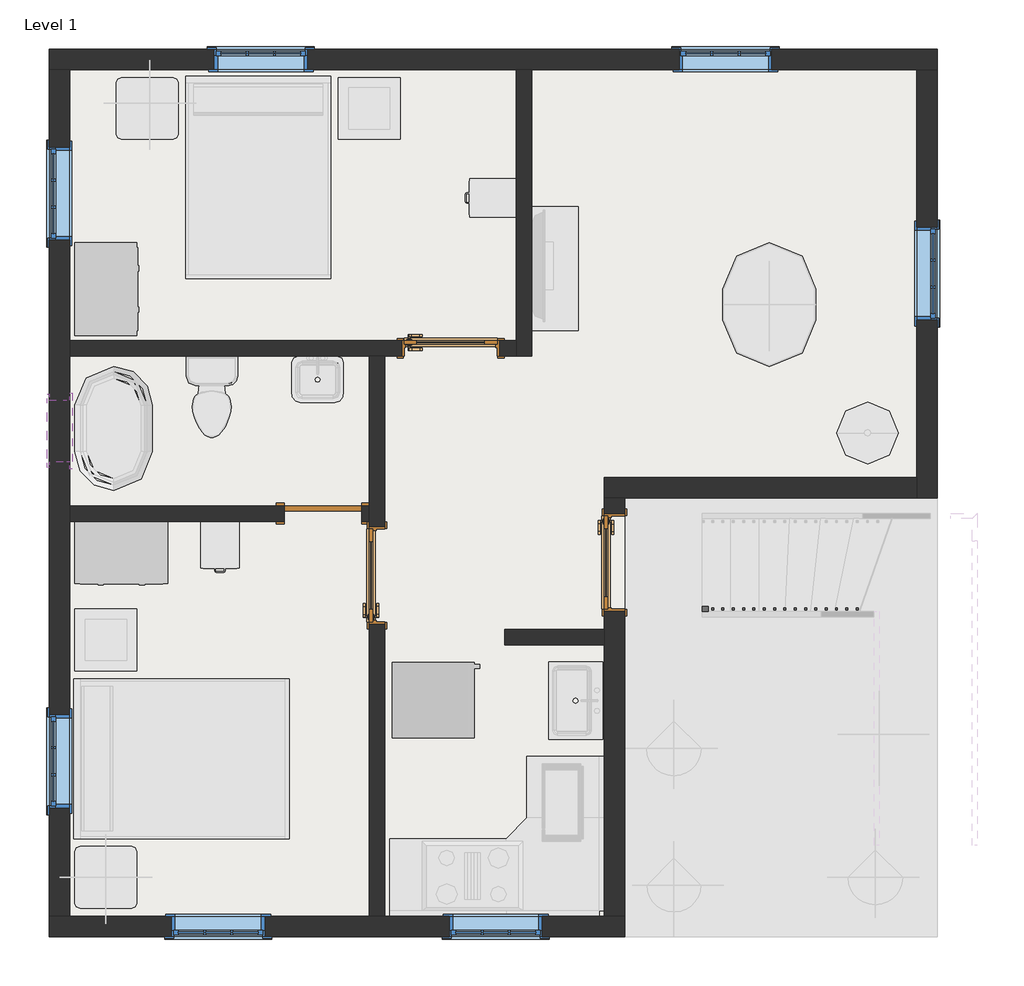
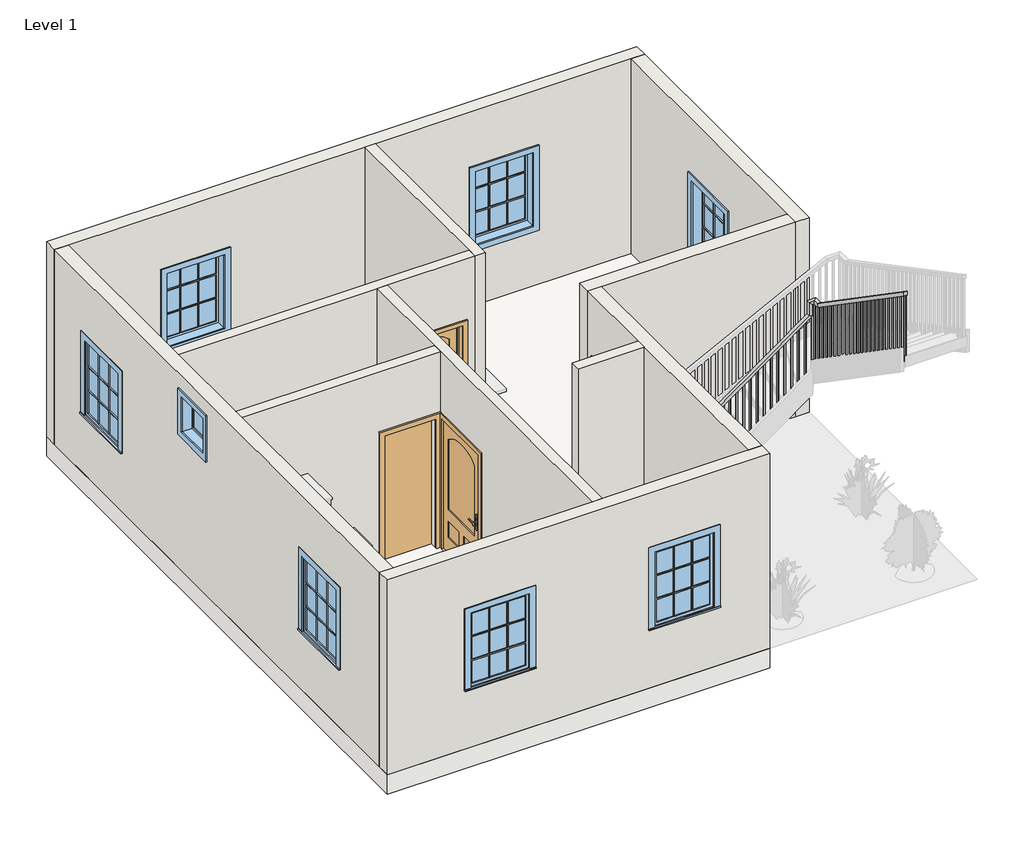
# One storey, part 1 of 2: 11 walls, 8 windows, 4 doors, 1 railing, 1 slab.
"""IFC4 building model written with IfcOpenShell, lengths in millimetres."""

from ifc_helpers import new_model, si_unit, frame, origin, origin_with_axes, place, context, project, spatial, polyline, outline, extrude, faceted_brep, transform, mapped, element, save
from components import door_5d363d20, door_1768e003, door_059fdd7e, window_29c06734, window_e41d21a6

model = new_model("IFC4")

# Units and contexts
model_context = context("Model", 3, world=origin())
ifc_project = project(units=[si_unit("LENGTHUNIT", "METRE", prefix="MILLI")], contexts=[model_context])

# Site, building, storey
site = spatial("IfcSite", under=ifc_project)
building = spatial("IfcBuilding", under=site)
storey = spatial("IfcBuildingStorey", under=building, Name="Level 1", Elevation=0.0)

# Doors
placement = place(None, origin())
door_shape = door_5d363d20(model_context)
element("IfcDoor", 1, ObjectType="36\" x 80\"", at=placement, inside=storey, context=model_context, shape_type="MappedRepresentation", body=[
    mapped(door_shape, transform((-9402.5770189, 12238.7273405, 0.0), x_axis=(-1.0, 0.0, 0.0), y_axis=(0.0, -1.0, 0.0), z_axis=(0.0, 0.0, 1.0))),
])
element("IfcDoor", 2, ObjectType="36\" x 80\"", at=placement, inside=storey, context=model_context, shape_type="MappedRepresentation", body=[
    mapped(door_shape, transform((-10129.6520189, 10000.3523405, 0.0), x_axis=(0.0, -1.0, 0.0), y_axis=(1.0, 0.0, 0.0), z_axis=(0.0, 0.0, 1.0))),
])
door_2_shape = door_1768e003(model_context)
element("IfcDoor", 3, ObjectType="36\" x 80\"", at=placement, inside=storey, context=model_context, shape_type="MappedRepresentation", body=[
    mapped(door_2_shape, transform((-7792.8520189, 10127.3523405, 0.0), x_axis=(0.0, 1.0, 0.0), y_axis=(-1.0, 0.0, 0.0), z_axis=(0.0, 0.0, 1.0))),
])
door_3_shape = door_059fdd7e(model_context)
element("IfcDoor", 4, ObjectType="Single-Flush : 30\" x 80\"", at=placement, inside=storey, context=model_context, shape_type="MappedRepresentation", body=[
    mapped(door_3_shape, transform((-10659.8770189, 10609.9523405, 0.0), x_axis=(1.0, 0.0, 0.0), y_axis=(0.0, 1.0, 0.0), z_axis=(0.0, 0.0, 1.0))),
])

# Railing
element("IfcRailing", 5, ObjectType="Handrail - Rectangular", at=placement, inside=storey, context=model_context, shape_type="SolidModel", body=[
    faceted_brep([(-6926.0770189, 9695.5523405, 1221.3337634), (-6926.0770189, 9695.5523405, 1158.7470985), (-6926.0770189, 9644.7523405, 1158.7470985), (-6926.0770189, 9644.7523405, 1221.3337634), (-5260.1400294, 9695.5523405, 2420.2016261), (-5209.3400294, 9695.5523405, 2394.1724587), (-5209.3400294, 9644.7523405, 2394.1724587), (-5260.1400294, 9644.7523405, 2420.2016261), (-5260.1400294, 9695.5523405, 2625.1172738), (-5209.3400294, 9695.5523405, 2574.3172738), (-5209.3400294, 9644.7523405, 2574.3172738), (-5260.1400294, 9644.7523405, 2625.1172738), (-5133.1400294, 9695.5523405, 2625.1172738), (-5133.1400294, 9695.5523405, 2574.3172738), (-5183.9400294, 9644.7523405, 2574.3172738), (-5183.9400294, 9644.7523405, 2625.1172738), (-5133.1400294, 9568.5523405, 2625.1172738), (-5133.1400294, 9552.7757051, 2574.3172738), (-5183.9400294, 9552.7757051, 2574.3172738), (-5183.9400294, 9568.5523405, 2625.1172738), (-5133.1400294, 7343.815351, 4154.4679017), (-5183.9400294, 7343.815351, 4154.4679017), (-5183.9400294, 7343.815351, 4092.8225715), (-5133.1400294, 7343.815351, 4092.8225715)], [[[0, 1, 2, 3]], [[1, 0, 4, 5]], [[2, 1, 5, 6]], [[3, 2, 6, 7]], [[0, 3, 7, 4]], [[5, 4, 8, 9]], [[6, 5, 9, 10]], [[7, 6, 10, 11]], [[4, 7, 11, 8]], [[9, 8, 12, 13]], [[10, 9, 13, 14]], [[11, 10, 14, 15]], [[8, 11, 15, 12]], [[13, 12, 16, 17]], [[14, 13, 17, 18]], [[15, 14, 18, 19]], [[12, 15, 19, 16]], [[20, 21, 22, 23]], [[17, 16, 20, 23]], [[18, 17, 23, 22]], [[19, 18, 22, 21]], [[16, 19, 21, 20]]]),
    extrude(outline(polyline([(7425.4273405, 4036.7200533), (7444.4773405, 4023.6245146), (7444.4773405, 3048.0), (7425.4273405, 3048.0), (7425.4273405, 4036.7200533)])), frame((-5168.0650294, 0.0, 0.0), z_axis=(1.0, 0.0, 0.0), x_axis=(0.0, 1.0, 0.0)), (0.0, 0.0, 1.0), 19.05),
    extrude(outline(polyline([(7527.0273405, 3966.87718), (7546.0773405, 3953.7816412), (7546.0773405, 3048.0), (7527.0273405, 3048.0), (7527.0273405, 3966.87718)])), frame((-5168.0650294, 0.0, 0.0), z_axis=(1.0, 0.0, 0.0), x_axis=(0.0, 1.0, 0.0)), (0.0, 0.0, 1.0), 19.05),
    extrude(outline(polyline([(7628.6273405, 3897.0343066), (7647.6773405, 3883.9387679), (7647.6773405, 2878.6666667), (7628.6273405, 2878.6666667), (7628.6273405, 3897.0343066)])), frame((-5168.0650294, 0.0, 0.0), z_axis=(1.0, 0.0, 0.0), x_axis=(0.0, 1.0, 0.0)), (0.0, 0.0, 1.0), 19.05),
    extrude(outline(polyline([(7730.2273405, 3827.1914333), (7749.2773405, 3814.0958945), (7749.2773405, 2878.6666667), (7730.2273405, 2878.6666667), (7730.2273405, 3827.1914333)])), frame((-5168.0650294, 0.0, 0.0), z_axis=(1.0, 0.0, 0.0), x_axis=(0.0, 1.0, 0.0)), (0.0, 0.0, 1.0), 19.05),
    extrude(outline(polyline([(7831.8273405, 3757.3485599), (7850.8773405, 3744.2530212), (7850.8773405, 2878.6666667), (7831.8273405, 2878.6666667), (7831.8273405, 3757.3485599)])), frame((-5168.0650294, 0.0, 0.0), z_axis=(1.0, 0.0, 0.0), x_axis=(0.0, 1.0, 0.0)), (0.0, 0.0, 1.0), 19.05),
    extrude(outline(polyline([(7933.4273405, 3687.5056866), (7952.4773405, 3674.4101478), (7952.4773405, 2709.3333333), (7933.4273405, 2709.3333333), (7933.4273405, 3687.5056866)])), frame((-5168.0650294, 0.0, 0.0), z_axis=(1.0, 0.0, 0.0), x_axis=(0.0, 1.0, 0.0)), (0.0, 0.0, 1.0), 19.05),
    extrude(outline(polyline([(8035.0273405, 3617.6628132), (8054.0773405, 3604.5672745), (8054.0773405, 2709.3333333), (8035.0273405, 2709.3333333), (8035.0273405, 3617.6628132)])), frame((-5168.0650294, 0.0, 0.0), z_axis=(1.0, 0.0, 0.0), x_axis=(0.0, 1.0, 0.0)), (0.0, 0.0, 1.0), 19.05),
    extrude(outline(polyline([(8136.6273405, 3547.8199399), (8155.6773405, 3534.7244011), (8155.6773405, 2709.3333333), (8136.6273405, 2709.3333333), (8136.6273405, 3547.8199399)])), frame((-5168.0650294, 0.0, 0.0), z_axis=(1.0, 0.0, 0.0), x_axis=(0.0, 1.0, 0.0)), (0.0, 0.0, 1.0), 19.05),
    extrude(outline(polyline([(8238.2273405, 3477.9770665), (8257.2773405, 3464.8815278), (8257.2773405, 2540.0), (8238.2273405, 2540.0), (8238.2273405, 3477.9770665)])), frame((-5168.0650294, 0.0, 0.0), z_axis=(1.0, 0.0, 0.0), x_axis=(0.0, 1.0, 0.0)), (0.0, 0.0, 1.0), 19.05),
    extrude(outline(polyline([(8339.8273405, 3408.1341932), (8358.8773405, 3395.0386544), (8358.8773405, 2540.0), (8339.8273405, 2540.0), (8339.8273405, 3408.1341932)])), frame((-5168.0650294, 0.0, 0.0), z_axis=(1.0, 0.0, 0.0), x_axis=(0.0, 1.0, 0.0)), (0.0, 0.0, 1.0), 19.05),
    extrude(outline(polyline([(8441.4273405, 3338.2913198), (8460.4773405, 3325.1957811), (8460.4773405, 2370.6666667), (8441.4273405, 2370.6666667), (8441.4273405, 3338.2913198)])), frame((-5168.0650294, 0.0, 0.0), z_axis=(1.0, 0.0, 0.0), x_axis=(0.0, 1.0, 0.0)), (0.0, 0.0, 1.0), 19.05),
    extrude(outline(polyline([(8543.0273405, 3268.4484465), (8562.0773405, 3255.3529077), (8562.0773405, 2370.6666667), (8543.0273405, 2370.6666667), (8543.0273405, 3268.4484465)])), frame((-5168.0650294, 0.0, 0.0), z_axis=(1.0, 0.0, 0.0), x_axis=(0.0, 1.0, 0.0)), (0.0, 0.0, 1.0), 19.05),
    extrude(outline(polyline([(8644.6273405, 3198.6055731), (8663.6773405, 3185.5100344), (8663.6773405, 2370.6666667), (8644.6273405, 2370.6666667), (8644.6273405, 3198.6055731)])), frame((-5168.0650294, 0.0, 0.0), z_axis=(1.0, 0.0, 0.0), x_axis=(0.0, 1.0, 0.0)), (0.0, 0.0, 1.0), 19.05),
    extrude(outline(polyline([(8746.2273405, 3128.7626998), (8765.2773405, 3115.667161), (8765.2773405, 2201.3333333), (8746.2273405, 2201.3333333), (8746.2273405, 3128.7626998)])), frame((-5168.0650294, 0.0, 0.0), z_axis=(1.0, 0.0, 0.0), x_axis=(0.0, 1.0, 0.0)), (0.0, 0.0, 1.0), 19.05),
    extrude(outline(polyline([(8847.8273405, 3058.9198264), (8866.8773405, 3045.8242877), (8866.8773405, 2201.3333333), (8847.8273405, 2201.3333333), (8847.8273405, 3058.9198264)])), frame((-5168.0650294, 0.0, 0.0), z_axis=(1.0, 0.0, 0.0), x_axis=(0.0, 1.0, 0.0)), (0.0, 0.0, 1.0), 19.05),
    extrude(outline(polyline([(8949.4273405, 2989.0769531), (8968.4773405, 2975.9814143), (8968.4773405, 2032.0), (8949.4273405, 2032.0), (8949.4273405, 2989.0769531)])), frame((-5168.0650294, 0.0, 0.0), z_axis=(1.0, 0.0, 0.0), x_axis=(0.0, 1.0, 0.0)), (0.0, 0.0, 1.0), 19.05),
    extrude(outline(polyline([(9051.0273405, 2919.2340797), (9070.0773405, 2906.138541), (9070.0773405, 2032.0), (9051.0273405, 2032.0), (9051.0273405, 2919.2340797)])), frame((-5168.0650294, 0.0, 0.0), z_axis=(1.0, 0.0, 0.0), x_axis=(0.0, 1.0, 0.0)), (0.0, 0.0, 1.0), 19.05),
    extrude(outline(polyline([(9152.6273405, 2849.3912064), (9171.6773405, 2836.2956676), (9171.6773405, 2032.0), (9152.6273405, 2032.0), (9152.6273405, 2849.3912064)])), frame((-5168.0650294, 0.0, 0.0), z_axis=(1.0, 0.0, 0.0), x_axis=(0.0, 1.0, 0.0)), (0.0, 0.0, 1.0), 19.05),
    extrude(outline(polyline([(9254.2273405, 2779.548333), (9273.2773405, 2766.4527943), (9273.2773405, 1862.6666667), (9254.2273405, 1862.6666667), (9254.2273405, 2779.548333)])), frame((-5168.0650294, 0.0, 0.0), z_axis=(1.0, 0.0, 0.0), x_axis=(0.0, 1.0, 0.0)), (0.0, 0.0, 1.0), 19.05),
    extrude(outline(polyline([(9355.8273405, 2709.7054597), (9374.8773405, 2696.6099209), (9374.8773405, 1862.6666667), (9355.8273405, 1862.6666667), (9355.8273405, 2709.7054597)])), frame((-5168.0650294, 0.0, 0.0), z_axis=(1.0, 0.0, 0.0), x_axis=(0.0, 1.0, 0.0)), (0.0, 0.0, 1.0), 19.05),
    extrude(outline(polyline([(9457.4273405, 2639.8625863), (9476.4773405, 2626.7670476), (9476.4773405, 1693.3333333), (9457.4273405, 1693.3333333), (9457.4273405, 2639.8625863)])), frame((-5168.0650294, 0.0, 0.0), z_axis=(1.0, 0.0, 0.0), x_axis=(0.0, 1.0, 0.0)), (0.0, 0.0, 1.0), 19.05),
    extrude(outline(polyline([(-5168.0650294, 9578.0773405), (-5149.0150294, 9578.0773405), (-5149.0150294, 9559.0273405), (-5168.0650294, 9559.0273405), (-5168.0650294, 9578.0773405)])), frame((0.0, 0.0, 1693.3333333), z_axis=(0.0, 0.0, 1.0), x_axis=(1.0, 0.0, 0.0)), (0.0, 0.0, 1.0), 880.9839405),
    extrude(outline(polyline([(2408.5565462, -5189.3520189), (2394.8474846, -5208.4020189), (1524.0, -5208.4020189), (1524.0, -5189.3520189), (2408.5565462, -5189.3520189)])), frame((0.0, 9660.6273405, 0.0), z_axis=(0.0, 1.0, 0.0), x_axis=(0.0, 0.0, 1.0)), (0.0, 0.0, 1.0), 19.05),
    extrude(outline(polyline([(2335.4415511, -5290.9520189), (2321.7324895, -5310.0020189), (1354.6666667, -5310.0020189), (1354.6666667, -5290.9520189), (2335.4415511, -5290.9520189)])), frame((0.0, 9660.6273405, 0.0), z_axis=(0.0, 1.0, 0.0), x_axis=(0.0, 0.0, 1.0)), (0.0, 0.0, 1.0), 19.05),
    extrude(outline(polyline([(2262.326556, -5392.5520189), (2248.6174944, -5411.6020189), (1185.3333333, -5411.6020189), (1185.3333333, -5392.5520189), (2262.326556, -5392.5520189)])), frame((0.0, 9660.6273405, 0.0), z_axis=(0.0, 1.0, 0.0), x_axis=(0.0, 0.0, 1.0)), (0.0, 0.0, 1.0), 19.05),
    extrude(outline(polyline([(2189.2115609, -5494.1520189), (2175.5024993, -5513.2020189), (1185.3333333, -5513.2020189), (1185.3333333, -5494.1520189), (2189.2115609, -5494.1520189)])), frame((0.0, 9660.6273405, 0.0), z_axis=(0.0, 1.0, 0.0), x_axis=(0.0, 0.0, 1.0)), (0.0, 0.0, 1.0), 19.05),
    extrude(outline(polyline([(2116.0965658, -5595.7520189), (2102.3875042, -5614.8020189), (1185.3333333, -5614.8020189), (1185.3333333, -5595.7520189), (2116.0965658, -5595.7520189)])), frame((0.0, 9660.6273405, 0.0), z_axis=(0.0, 1.0, 0.0), x_axis=(0.0, 0.0, 1.0)), (0.0, 0.0, 1.0), 19.05),
    extrude(outline(polyline([(2042.9815706, -5697.3520189), (2029.2725091, -5716.4020189), (1016.0, -5716.4020189), (1016.0, -5697.3520189), (2042.9815706, -5697.3520189)])), frame((0.0, 9660.6273405, 0.0), z_axis=(0.0, 1.0, 0.0), x_axis=(0.0, 0.0, 1.0)), (0.0, 0.0, 1.0), 19.05),
    extrude(outline(polyline([(1969.8665755, -5798.9520189), (1956.1575139, -5818.0020189), (1016.0, -5818.0020189), (1016.0, -5798.9520189), (1969.8665755, -5798.9520189)])), frame((0.0, 9660.6273405, 0.0), z_axis=(0.0, 1.0, 0.0), x_axis=(0.0, 0.0, 1.0)), (0.0, 0.0, 1.0), 19.05),
    extrude(outline(polyline([(1896.7515804, -5900.5520189), (1883.0425188, -5919.6020189), (846.6666667, -5919.6020189), (846.6666667, -5900.5520189), (1896.7515804, -5900.5520189)])), frame((0.0, 9660.6273405, 0.0), z_axis=(0.0, 1.0, 0.0), x_axis=(0.0, 0.0, 1.0)), (0.0, 0.0, 1.0), 19.05),
    extrude(outline(polyline([(1823.6365853, -6002.1520189), (1809.9275237, -6021.2020189), (846.6666667, -6021.2020189), (846.6666667, -6002.1520189), (1823.6365853, -6002.1520189)])), frame((0.0, 9660.6273405, 0.0), z_axis=(0.0, 1.0, 0.0), x_axis=(0.0, 0.0, 1.0)), (0.0, 0.0, 1.0), 19.05),
    extrude(outline(polyline([(1750.5215902, -6103.7520189), (1736.8125286, -6122.8020189), (677.3333333, -6122.8020189), (677.3333333, -6103.7520189), (1750.5215902, -6103.7520189)])), frame((0.0, 9660.6273405, 0.0), z_axis=(0.0, 1.0, 0.0), x_axis=(0.0, 0.0, 1.0)), (0.0, 0.0, 1.0), 19.05),
    extrude(outline(polyline([(1677.4065951, -6205.3520189), (1663.6975335, -6224.4020189), (677.3333333, -6224.4020189), (677.3333333, -6205.3520189), (1677.4065951, -6205.3520189)])), frame((0.0, 9660.6273405, 0.0), z_axis=(0.0, 1.0, 0.0), x_axis=(0.0, 0.0, 1.0)), (0.0, 0.0, 1.0), 19.05),
    extrude(outline(polyline([(1604.2916, -6306.9520189), (1590.5825384, -6326.0020189), (677.3333333, -6326.0020189), (677.3333333, -6306.9520189), (1604.2916, -6306.9520189)])), frame((0.0, 9660.6273405, 0.0), z_axis=(0.0, 1.0, 0.0), x_axis=(0.0, 0.0, 1.0)), (0.0, 0.0, 1.0), 19.05),
    extrude(outline(polyline([(1531.1766049, -6408.5520189), (1517.4675433, -6427.6020189), (508.0, -6427.6020189), (508.0, -6408.5520189), (1531.1766049, -6408.5520189)])), frame((0.0, 9660.6273405, 0.0), z_axis=(0.0, 1.0, 0.0), x_axis=(0.0, 0.0, 1.0)), (0.0, 0.0, 1.0), 19.05),
    extrude(outline(polyline([(1458.0616097, -6510.1520189), (1444.3525482, -6529.2020189), (508.0, -6529.2020189), (508.0, -6510.1520189), (1458.0616097, -6510.1520189)])), frame((0.0, 9660.6273405, 0.0), z_axis=(0.0, 1.0, 0.0), x_axis=(0.0, 0.0, 1.0)), (0.0, 0.0, 1.0), 19.05),
    extrude(outline(polyline([(1384.9466146, -6611.7520189), (1371.2375531, -6630.8020189), (508.0, -6630.8020189), (508.0, -6611.7520189), (1384.9466146, -6611.7520189)])), frame((0.0, 9660.6273405, 0.0), z_axis=(0.0, 1.0, 0.0), x_axis=(0.0, 0.0, 1.0)), (0.0, 0.0, 1.0), 19.05),
    extrude(outline(polyline([(1311.8316195, -6713.3520189), (1298.1225579, -6732.4020189), (338.6666667, -6732.4020189), (338.6666667, -6713.3520189), (1311.8316195, -6713.3520189)])), frame((0.0, 9660.6273405, 0.0), z_axis=(0.0, 1.0, 0.0), x_axis=(0.0, 0.0, 1.0)), (0.0, 0.0, 1.0), 19.05),
    extrude(outline(polyline([(1238.7166244, -6814.9520189), (1225.0075628, -6834.0020189), (338.6666667, -6834.0020189), (338.6666667, -6814.9520189), (1238.7166244, -6814.9520189)])), frame((0.0, 9660.6273405, 0.0), z_axis=(0.0, 1.0, 0.0), x_axis=(0.0, 0.0, 1.0)), (0.0, 0.0, 1.0), 19.05),
    extrude(outline(polyline([(-5168.0650294, 9679.6773405), (-5149.0150294, 9679.6773405), (-5149.0150294, 9660.6273405), (-5168.0650294, 9660.6273405), (-5168.0650294, 9679.6773405)])), frame((0.0, 0.0, 1524.0), z_axis=(0.0, 0.0, 1.0), x_axis=(1.0, 0.0, 0.0)), (0.0, 0.0, 1.0), 1050.3172738),
    extrude(outline(polyline([(7343.815351, 4092.8225715), (7362.865351, 4079.7270327), (7362.865351, 3048.0), (7343.815351, 3048.0), (7343.815351, 4092.8225715)])), frame((-5168.0650294, 0.0, 0.0), z_axis=(1.0, 0.0, 0.0), x_axis=(0.0, 1.0, 0.0)), (0.0, 0.0, 1.0), 19.05),
    extrude(outline(polyline([(1172.4561601, -6907.0270189), (1158.7470985, -6926.0770189), (338.6666667, -6926.0770189), (338.6666667, -6907.0270189), (1172.4561601, -6907.0270189)])), frame((0.0, 9660.6273405, 0.0), z_axis=(0.0, 1.0, 0.0), x_axis=(0.0, 0.0, 1.0)), (0.0, 0.0, 1.0), 19.05),
])

# Slab
element("IfcSlab", 6, ObjectType="Generic - 12\"", at=placement, inside=storey, context=model_context, shape_type="SweptSolid", body=[
    extrude(outline(polyline([(-4614.6770189, 15181.9523405), (-4614.6770189, 10762.3523405), (-7688.0770189, 10762.3523405), (-7688.0770189, 6444.3523405), (-13352.2770189, 6444.3523405), (-13352.2770189, 15181.9523405), (-4614.6770189, 15181.9523405)])), frame((0.0, 0.0, -304.8), z_axis=(0.0, 0.0, 1.0), x_axis=(1.0, 0.0, 0.0)), (0.0, 0.0, 1.0), 304.8),
])

# Walls
element("IfcWall", 7, ObjectType="Generic - 8\"", at=placement, inside=storey, context=model_context, shape_type="Brep", body=[
    faceted_brep([(-13352.2770189, 14978.7523405, 0.0), (-13149.0770189, 14978.7523405, 0.0), (-8754.8770189, 14978.7523405, 0.0), (-8602.4770189, 14978.7523405, 0.0), (-4817.8770189, 14978.7523405, 0.0), (-4614.6770189, 14978.7523405, 0.0), (-4614.6770189, 14978.7523405, 3048.0), (-4817.8770189, 14978.7523405, 3048.0), (-8602.4770189, 14978.7523405, 3048.0), (-8754.8770189, 14978.7523405, 3048.0), (-13149.0770189, 14978.7523405, 3048.0), (-13352.2770189, 14978.7523405, 3048.0), (-10812.2770189, 14978.7523405, 2133.6), (-10812.2770189, 14978.7523405, 914.4), (-11726.6770189, 14978.7523405, 914.4), (-11726.6770189, 14978.7523405, 2133.6), (-6240.2770189, 14978.7523405, 2133.6), (-6240.2770189, 14978.7523405, 914.4), (-7154.6770189, 14978.7523405, 914.4), (-7154.6770189, 14978.7523405, 2133.6), (-13352.2770189, 15181.9523405, 0.0), (-13352.2770189, 15181.9523405, 3048.0), (-4614.6770189, 15181.9523405, 3048.0), (-4614.6770189, 15181.9523405, 0.0), (-10812.2770189, 15181.9523405, 2133.6), (-11726.6770189, 15181.9523405, 2133.6), (-11726.6770189, 15181.9523405, 914.4), (-10812.2770189, 15181.9523405, 914.4), (-6240.2770189, 15181.9523405, 2133.6), (-7154.6770189, 15181.9523405, 2133.6), (-7154.6770189, 15181.9523405, 914.4), (-6240.2770189, 15181.9523405, 914.4)], [[[0, 1, 2, 3, 4, 5, 6, 7, 8, 9, 10, 11], [12, 13, 14, 15], [16, 17, 18, 19]], [[20, 21, 22, 23], [24, 25, 26, 27], [28, 29, 30, 31]], [[5, 4, 3, 2, 1, 0, 20, 23]], [[6, 5, 23, 22]], [[0, 11, 21, 20]], [[13, 12, 24, 27]], [[14, 13, 27, 26]], [[15, 14, 26, 25]], [[12, 15, 25, 24]], [[17, 16, 28, 31]], [[18, 17, 31, 30]], [[19, 18, 30, 29]], [[16, 19, 29, 28]], [[11, 10, 9, 8, 7, 6, 22, 21]]]),
])
element("IfcWall", 8, ObjectType="Generic - 8\"", at=placement, inside=storey, context=model_context, shape_type="Brep", body=[
    faceted_brep([(-4817.8770189, 14978.7523405, 0.0), (-4817.8770189, 10965.5523405, 0.0), (-4817.8770189, 10762.3523405, 0.0), (-4817.8770189, 10762.3523405, 3048.0), (-4817.8770189, 10965.5523405, 3048.0), (-4817.8770189, 14978.7523405, 3048.0), (-4817.8770189, 12514.9523405, 2133.6), (-4817.8770189, 12514.9523405, 914.4), (-4817.8770189, 13429.3523405, 914.4), (-4817.8770189, 13429.3523405, 2133.6), (-4614.6770189, 14978.7523405, 0.0), (-4614.6770189, 14978.7523405, 3048.0), (-4614.6770189, 10762.3523405, 3048.0), (-4614.6770189, 10762.3523405, 0.0), (-4614.6770189, 12514.9523405, 2133.6), (-4614.6770189, 13429.3523405, 2133.6), (-4614.6770189, 13429.3523405, 914.4), (-4614.6770189, 12514.9523405, 914.4)], [[[0, 1, 2, 3, 4, 5], [6, 7, 8, 9]], [[10, 11, 12, 13], [14, 15, 16, 17]], [[2, 1, 0, 10, 13]], [[0, 5, 11, 10]], [[3, 2, 13, 12]], [[7, 6, 14, 17]], [[8, 7, 17, 16]], [[9, 8, 16, 15]], [[6, 9, 15, 14]], [[5, 4, 3, 12, 11]]]),
])
element("IfcWall", 9, ObjectType="Generic - 8\"", at=placement, inside=storey, context=model_context, shape_type="Brep", body=[
    faceted_brep([(-13149.0770189, 6647.5523405, 0.0), (-13149.0770189, 10533.7523405, 0.0), (-13149.0770189, 10686.1523405, 0.0), (-13149.0770189, 12159.3523405, 0.0), (-13149.0770189, 12311.7523405, 0.0), (-13149.0770189, 14978.7523405, 0.0), (-13149.0770189, 14978.7523405, 3048.0), (-13149.0770189, 12311.7523405, 3048.0), (-13149.0770189, 12159.3523405, 3048.0), (-13149.0770189, 10686.1523405, 3048.0), (-13149.0770189, 10533.7523405, 3048.0), (-13149.0770189, 6647.5523405, 3048.0), (-13149.0770189, 14216.7523405, 2133.6), (-13149.0770189, 14216.7523405, 914.4), (-13149.0770189, 13302.3523405, 914.4), (-13149.0770189, 13302.3523405, 2133.6), (-13149.0770189, 8628.7523405, 2133.6), (-13149.0770189, 8628.7523405, 914.4), (-13149.0770189, 7714.3523405, 914.4), (-13149.0770189, 7714.3523405, 2133.6), (-13149.0770189, 11117.9523405, 2768.6), (-13149.0770189, 11727.5523405, 2768.6), (-13149.0770189, 11727.5523405, 2159.0), (-13149.0770189, 11117.9523405, 2159.0), (-13352.2770189, 6647.5523405, 0.0), (-13352.2770189, 6647.5523405, 3048.0), (-13352.2770189, 14978.7523405, 3048.0), (-13352.2770189, 14978.7523405, 0.0), (-13352.2770189, 14216.7523405, 2133.6), (-13352.2770189, 13302.3523405, 2133.6), (-13352.2770189, 13302.3523405, 914.4), (-13352.2770189, 14216.7523405, 914.4), (-13352.2770189, 8628.7523405, 2133.6), (-13352.2770189, 7714.3523405, 2133.6), (-13352.2770189, 7714.3523405, 914.4), (-13352.2770189, 8628.7523405, 914.4), (-13352.2770189, 11117.9523405, 2768.6), (-13352.2770189, 11117.9523405, 2159.0), (-13352.2770189, 11727.5523405, 2159.0), (-13352.2770189, 11727.5523405, 2768.6)], [[[0, 1, 2, 3, 4, 5, 6, 7, 8, 9, 10, 11], [12, 13, 14, 15], [16, 17, 18, 19], [20, 21, 22, 23]], [[24, 25, 26, 27], [28, 29, 30, 31], [32, 33, 34, 35], [36, 37, 38, 39]], [[5, 4, 3, 2, 1, 0, 24, 27]], [[6, 5, 27, 26]], [[0, 11, 25, 24]], [[13, 12, 28, 31]], [[14, 13, 31, 30]], [[15, 14, 30, 29]], [[12, 15, 29, 28]], [[17, 16, 32, 35]], [[18, 17, 35, 34]], [[19, 18, 34, 33]], [[16, 19, 33, 32]], [[37, 36, 20, 23]], [[38, 37, 23, 22]], [[39, 38, 22, 21]], [[36, 39, 21, 20]], [[11, 10, 9, 8, 7, 6, 26, 25]]]),
])
element("IfcWall", 10, ObjectType="Generic - 8\"", at=placement, inside=storey, context=model_context, shape_type="Brep", body=[
    faceted_brep([(-7891.2770189, 6647.5523405, 0.0), (-7891.2770189, 6647.5523405, 3048.0), (-7891.2770189, 9314.5523405, 3048.0), (-7891.2770189, 9466.9523405, 3048.0), (-7891.2770189, 10762.3523405, 3048.0), (-7891.2770189, 10762.3523405, 0.0), (-7891.2770189, 10609.9523405, 0.0), (-7891.2770189, 10609.9523405, 2057.4), (-7891.2770189, 9644.7523405, 2057.4), (-7891.2770189, 9644.7523405, 0.0), (-7891.2770189, 9466.9523405, 0.0), (-7891.2770189, 9314.5523405, 0.0), (-7688.0770189, 6647.5523405, 3048.0), (-7688.0770189, 6647.5523405, 0.0), (-7688.0770189, 9644.7523405, 0.0), (-7688.0770189, 9644.7523405, 2057.4), (-7688.0770189, 10609.9523405, 2057.4), (-7688.0770189, 10609.9523405, 0.0), (-7688.0770189, 10762.3523405, 0.0), (-7688.0770189, 10762.3523405, 3048.0)], [[[0, 1, 2, 3, 4, 5, 6, 7, 8, 9, 10, 11]], [[12, 13, 14, 15, 16, 17, 18, 19]], [[13, 0, 11, 10, 9, 14]], [[5, 18, 17, 6]], [[1, 0, 13, 12]], [[5, 4, 19, 18]], [[16, 7, 6, 17]], [[7, 16, 15, 8]], [[8, 15, 14, 9]], [[4, 3, 2, 1, 12, 19]]]),
])
element("IfcWall", 11, ObjectType="Generic - 8\"", at=placement, inside=storey, context=model_context, shape_type="Brep", body=[
    faceted_brep([(-7891.2770189, 10762.3523405, 0.0), (-7688.0770189, 10762.3523405, 0.0), (-4817.8770189, 10762.3523405, 0.0), (-4817.8770189, 10762.3523405, 3048.0), (-7688.0770189, 10762.3523405, 3048.0), (-7891.2770189, 10762.3523405, 3048.0), (-7891.2770189, 10965.5523405, 0.0), (-7891.2770189, 10965.5523405, 3048.0), (-4817.8770189, 10965.5523405, 3048.0), (-4817.8770189, 10965.5523405, 0.0)], [[[0, 1, 2, 3, 4, 5]], [[6, 7, 8, 9]], [[2, 1, 0, 6, 9]], [[3, 2, 9, 8]], [[0, 5, 7, 6]], [[5, 4, 3, 8, 7]]]),
])
element("IfcWall", 12, ObjectType="Generic - 8\"", at=placement, inside=storey, context=model_context, shape_type="Brep", body=[
    faceted_brep([(-7688.0770189, 6647.5523405, 0.0), (-7891.2770189, 6647.5523405, 0.0), (-10050.2770189, 6647.5523405, 0.0), (-10202.6770189, 6647.5523405, 0.0), (-13149.0770189, 6647.5523405, 0.0), (-13352.2770189, 6647.5523405, 0.0), (-13352.2770189, 6647.5523405, 3048.0), (-13149.0770189, 6647.5523405, 3048.0), (-10202.6770189, 6647.5523405, 3048.0), (-10050.2770189, 6647.5523405, 3048.0), (-7891.2770189, 6647.5523405, 3048.0), (-7688.0770189, 6647.5523405, 3048.0), (-12145.7770189, 6647.5523405, 2133.6), (-12145.7770189, 6647.5523405, 914.4), (-11231.3770189, 6647.5523405, 914.4), (-11231.3770189, 6647.5523405, 2133.6), (-9415.2770189, 6647.5523405, 2133.6), (-9415.2770189, 6647.5523405, 914.4), (-8500.8770189, 6647.5523405, 914.4), (-8500.8770189, 6647.5523405, 2133.6), (-7688.0770189, 6444.3523405, 0.0), (-7688.0770189, 6444.3523405, 3048.0), (-13352.2770189, 6444.3523405, 3048.0), (-13352.2770189, 6444.3523405, 0.0), (-12145.7770189, 6444.3523405, 2133.6), (-11231.3770189, 6444.3523405, 2133.6), (-11231.3770189, 6444.3523405, 914.4), (-12145.7770189, 6444.3523405, 914.4), (-9415.2770189, 6444.3523405, 2133.6), (-8500.8770189, 6444.3523405, 2133.6), (-8500.8770189, 6444.3523405, 914.4), (-9415.2770189, 6444.3523405, 914.4)], [[[0, 1, 2, 3, 4, 5, 6, 7, 8, 9, 10, 11], [12, 13, 14, 15], [16, 17, 18, 19]], [[20, 21, 22, 23], [24, 25, 26, 27], [28, 29, 30, 31]], [[5, 4, 3, 2, 1, 0, 20, 23]], [[6, 5, 23, 22]], [[0, 11, 21, 20]], [[13, 12, 24, 27]], [[14, 13, 27, 26]], [[15, 14, 26, 25]], [[12, 15, 25, 24]], [[17, 16, 28, 31]], [[18, 17, 31, 30]], [[19, 18, 30, 29]], [[16, 19, 29, 28]], [[11, 10, 9, 8, 7, 6, 22, 21]]]),
])
element("IfcWall", 13, ObjectType="INNER 6\"", at=placement, inside=storey, context=model_context, shape_type="Brep", body=[
    faceted_brep([(-8754.8770189, 14978.7523405, 0.0), (-8754.8770189, 12311.7523405, 0.0), (-8754.8770189, 12159.3523405, 0.0), (-8754.8770189, 12159.3523405, 3048.0), (-8754.8770189, 12311.7523405, 3048.0), (-8754.8770189, 14978.7523405, 3048.0), (-8602.4770189, 14978.7523405, 0.0), (-8602.4770189, 14978.7523405, 3048.0), (-8602.4770189, 12159.3523405, 3048.0), (-8602.4770189, 12159.3523405, 0.0)], [[[0, 1, 2, 3, 4, 5]], [[6, 7, 8, 9]], [[2, 1, 0, 6, 9]], [[0, 5, 7, 6]], [[3, 2, 9, 8]], [[5, 4, 3, 8, 7]]]),
])
element("IfcWall", 14, ObjectType="INNER 6\"", at=placement, inside=storey, context=model_context, shape_type="Brep", body=[
    faceted_brep([(-8754.8770189, 12311.7523405, 3048.0), (-8754.8770189, 12311.7523405, 0.0), (-8919.9770189, 12311.7523405, 0.0), (-8919.9770189, 12311.7523405, 2057.4), (-9885.1770189, 12311.7523405, 2057.4), (-9885.1770189, 12311.7523405, 0.0), (-13149.0770189, 12311.7523405, 0.0), (-13149.0770189, 12311.7523405, 3048.0), (-8754.8770189, 12159.3523405, 0.0), (-8754.8770189, 12159.3523405, 3048.0), (-10050.2770189, 12159.3523405, 3048.0), (-10202.6770189, 12159.3523405, 3048.0), (-13149.0770189, 12159.3523405, 3048.0), (-13149.0770189, 12159.3523405, 0.0), (-10202.6770189, 12159.3523405, 0.0), (-10050.2770189, 12159.3523405, 0.0), (-9885.1770189, 12159.3523405, 0.0), (-9885.1770189, 12159.3523405, 2057.4), (-8919.9770189, 12159.3523405, 2057.4), (-8919.9770189, 12159.3523405, 0.0)], [[[0, 1, 2, 3, 4, 5, 6, 7]], [[8, 9, 10, 11, 12, 13, 14, 15, 16, 17, 18, 19]], [[1, 8, 19, 2]], [[13, 6, 5, 16, 15, 14]], [[1, 0, 9, 8]], [[7, 6, 13, 12]], [[4, 17, 16, 5]], [[17, 4, 3, 18]], [[18, 3, 2, 19]], [[0, 7, 12, 11, 10, 9]]]),
])
element("IfcWall", 15, ObjectType="INNER 6\"", at=placement, inside=storey, context=model_context, shape_type="Brep", body=[
    faceted_brep([(-10202.6770189, 12159.3523405, 3048.0), (-10202.6770189, 12159.3523405, 0.0), (-10202.6770189, 10686.1523405, 0.0), (-10202.6770189, 10533.7523405, 0.0), (-10202.6770189, 10482.9523405, 0.0), (-10202.6770189, 10482.9523405, 2057.4), (-10202.6770189, 9517.7523405, 2057.4), (-10202.6770189, 9517.7523405, 0.0), (-10202.6770189, 6647.5523405, 0.0), (-10202.6770189, 6647.5523405, 3048.0), (-10202.6770189, 10533.7523405, 3048.0), (-10202.6770189, 10686.1523405, 3048.0), (-10050.2770189, 12159.3523405, 0.0), (-10050.2770189, 12159.3523405, 3048.0), (-10050.2770189, 6647.5523405, 3048.0), (-10050.2770189, 6647.5523405, 0.0), (-10050.2770189, 9517.7523405, 0.0), (-10050.2770189, 9517.7523405, 2057.4), (-10050.2770189, 10482.9523405, 2057.4), (-10050.2770189, 10482.9523405, 0.0)], [[[0, 1, 2, 3, 4, 5, 6, 7, 8, 9, 10, 11]], [[12, 13, 14, 15, 16, 17, 18, 19]], [[1, 12, 19, 4, 3, 2]], [[15, 8, 7, 16]], [[1, 0, 13, 12]], [[9, 8, 15, 14]], [[6, 17, 16, 7]], [[17, 6, 5, 18]], [[18, 5, 4, 19]], [[0, 11, 10, 9, 14, 13]]]),
])
element("IfcWall", 16, ObjectType="INNER 6\"", at=placement, inside=storey, context=model_context, shape_type="SweptSolid", body=[
    extrude(outline(polyline([(2032.0, -10278.8770189), (0.0, -10278.8770189), (0.0, -10202.6770189), (3048.0, -10202.6770189), (3048.0, -13149.0770189), (0.0, -13149.0770189), (0.0, -11040.8770189), (2032.0, -11040.8770189), (2032.0, -10278.8770189)])), frame((0.0, 10533.7523405, 0.0), z_axis=(0.0, 1.0, 0.0), x_axis=(0.0, 0.0, 1.0)), (0.0, 0.0, 1.0), 152.4),
])
element("IfcWall", 17, ObjectType="INNER 6\"", at=placement, inside=storey, context=model_context, shape_type="SweptSolid", body=[
    extrude(outline(polyline([(-7891.2770189, 9314.5523405), (-8869.1770189, 9314.5523405), (-8869.1770189, 9466.9523405), (-7891.2770189, 9466.9523405), (-7891.2770189, 9314.5523405)])), origin_with_axes(), (0.0, 0.0, 1.0), 3048.0),
])

# Windows
window_shape = window_29c06734(model_context)
element("IfcWindow", 18, ObjectType="Casement 3x3 with Trim : 36\" x 48\"", at=placement, inside=storey, context=model_context, shape_type="MappedRepresentation", body=[
    mapped(window_shape, transform((-11269.4770189, 15080.3523405, 0.0), x_axis=(1.0, 0.0, 0.0), y_axis=(0.0, 1.0, 0.0), z_axis=(0.0, 0.0, 1.0))),
])
element("IfcWindow", 19, ObjectType="Casement 3x3 with Trim : 36\" x 48\"", at=placement, inside=storey, context=model_context, shape_type="MappedRepresentation", body=[
    mapped(window_shape, transform((-13250.6770189, 13759.5523405, 0.0), x_axis=(0.0, 1.0, 0.0), y_axis=(-1.0, 0.0, 0.0), z_axis=(0.0, 0.0, 1.0))),
])
element("IfcWindow", 20, ObjectType="Casement 3x3 with Trim : 36\" x 48\"", at=placement, inside=storey, context=model_context, shape_type="MappedRepresentation", body=[
    mapped(window_shape, transform((-11688.5770189, 6545.9523405, 0.0), x_axis=(-1.0, 0.0, 0.0), y_axis=(0.0, -1.0, 0.0), z_axis=(0.0, 0.0, 1.0))),
])
element("IfcWindow", 21, ObjectType="Casement 3x3 with Trim : 36\" x 48\"", at=placement, inside=storey, context=model_context, shape_type="MappedRepresentation", body=[
    mapped(window_shape, transform((-13250.6770189, 8171.5523405, 0.0), x_axis=(0.0, 1.0, 0.0), y_axis=(-1.0, 0.0, 0.0), z_axis=(0.0, 0.0, 1.0))),
])
element("IfcWindow", 22, ObjectType="Casement 3x3 with Trim : 36\" x 48\"", at=placement, inside=storey, context=model_context, shape_type="MappedRepresentation", body=[
    mapped(window_shape, transform((-8958.0770189, 6545.9523405, 0.0), x_axis=(-1.0, 0.0, 0.0), y_axis=(0.0, -1.0, 0.0), z_axis=(0.0, 0.0, 1.0))),
])
element("IfcWindow", 23, ObjectType="Casement 3x3 with Trim : 36\" x 48\"", at=placement, inside=storey, context=model_context, shape_type="MappedRepresentation", body=[
    mapped(window_shape, transform((-6697.4770189, 15080.3523405, 0.0), x_axis=(1.0, 0.0, 0.0), y_axis=(0.0, 1.0, 0.0), z_axis=(0.0, 0.0, 1.0))),
])
element("IfcWindow", 24, ObjectType="Casement 3x3 with Trim : 36\" x 48\"", at=placement, inside=storey, context=model_context, shape_type="MappedRepresentation", body=[
    mapped(window_shape, transform((-4716.2770189, 12972.1523405, 0.0), x_axis=(0.0, -1.0, 0.0), y_axis=(1.0, 0.0, 0.0), z_axis=(0.0, 0.0, 1.0))),
])
window_2_shape = window_e41d21a6(model_context)
element("IfcWindow", 25, ObjectType="Transom with Trim : 24\" x 24\"", at=placement, inside=storey, context=model_context, shape_type="MappedRepresentation", body=[
    mapped(window_2_shape, transform((-13250.6770189, 11384.6523405, 0.0), x_axis=(0.0, -1.0, 0.0), y_axis=(1.0, 0.0, 0.0), z_axis=(0.0, 0.0, 1.0))),
])

save(model, "model.ifc")

# Revit data of these elements
# Type "36\" x 80\""
#   Type Mark = "8"
#   Assembly Code = "B2030100"
#   Analytic Construction = "French door, wood frame with single glass"
#   Threshold Offset [instance default] = 0' - 0 1/2"
#   Thickness = 0' - 1 3/8"
#   Thermal Resistance (R) = 1.0696 (h·ft²·°F)/BTU
#   Swing Angle [instance default] = 90.00°
#   Stiles = 0' - 4 3/4"
#   Rough Width = 3' - 2"
#   Rough Height = 6' - 9"
#   Radius = 1' - 8.05625"
#   Lock Rail = 0' - 7 1/8"
#   Height = 6' - 8"
#   Width = 3' - 0"
#   Heat Transfer Coefficient (U) = 0.9350 BTU/(h·ft²·°F)
#   Door Offset [instance default] = 0' - 0"
#   Bottom Rail = 0' - 9 1/2"
#   Threshold [instance default] = yes
#   Function = 1
#   Exterior Trim [instance default] = yes
#   Trim Material = Cherry
#   Threshold Material = Cherry
#   Panel Material = Cherry
#   Glazing = Glass
#   Frame Material = Cherry
#   Door Handle Material = Aluminum
#   Visual Light Transmittance = 0
#   Solar Heat Gain Coefficient = 0
#   Wall Closure = (empty or 0)
#   Construction Type = (empty or 0)
# Type "Single-Flush : 30\" x 80\""
#   Type Mark = "5"
#   Construction Type Id = "MDOOR"
#   Assembly Code = "C1020"
#   Analytic Construction = "Metal"
#   Thickness = 0' - 2"
#   Heat Transfer Coefficient (U) = 0.651978 BTU/(h·ft²·°F)
#   Height = 6' - 8"
#   Trim Projection Ext = 0' - 1"
#   Trim Projection Int = 0' - 1"
#   Trim Width = 0' - 3"
#   Width = 2' - 6"
#   Define Thermal Properties by = 1
#   Door Material = Door - Panel
#   Frame Material = Door - Frame
#   Visual Light Transmittance = 0
#   Solar Heat Gain Coefficient = 0
#   Function = (empty or 0)
#   Wall Closure = (empty or 0)
# Type "Handrail - Rectangular"
#   Assembly Code = "C2010400"
#   built-in parameter 1008612 = 0.0416667 (stored number, unit not read)
#   built-in parameter 1008611 = 0.0416667 (stored number, unit not read)
#   built-in parameter 1008609 = 0.333333 (stored number, unit not read)
#   built-in parameter 1008604 = 0.166667 (stored number, unit not read)
#   built-in parameter 1008603 = 0.166667 (stored number, unit not read)
#   Railing Height = 3' - 0"
#   built-in parameter 1008630 = 2
#   built-in parameter 1008610 = 2
#   built-in parameter 1008618 = Baluster - Square : 3/4"
# Type "Generic - 12\""
#   Assembly Code = "B1010"
#   Function = 0
#   Layers, outside or top first: 1' - 0" no material (function 1)
# Type "Generic - 8\""
#   Assembly Code = "B2010"
#   Layers, outside or top first: 0' - 8" "Brick, Common" (function 1)
# Type "INNER 6\""
#   Assembly Code = "B2010"
#   Layers, outside or top first: 0' - 6" "Brick, Common" (function 1)
# Type "Casement 3x3 with Trim : 36\" x 48\""
#   Type Mark = "10"
#   Construction Type Id = "GSP4R"
#   Assembly Code = "B2020100"
#   Analytic Construction = "1/8 in Pilkington single glazing"
#   Visual Light Transmittance = 0.9
#   Solar Heat Gain Coefficient = 0.78
#   Heat Transfer Coefficient (U) = 0.6496 BTU/(h·ft²·°F)
#   Height = 4' - 0"
#   Default Sill Height = 3' - 0"
#   Trim Projection - Ext. = 0' - 0 1/2"
#   Trim Projection - Int. = 0' - 0 3/4"
#   Trim Width - Exterior = 0' - 3 1/2"
#   Trim Width - Interior = 0' - 3 1/2"
#   Width = 3' - 0"
#   Window Inset = 0' - 0 3/4"
#   Define Thermal Properties by = 1
#   Glass Pane Material = Glass
#   Sash Material = Sash
#   Trim Exterior Material = Trim
#   Trim Interior Material = Trim
#   Wall Closure = (empty or 0)
# Type "Transom with Trim : 24\" x 24\""
#   Type Mark = "13"
#   Construction Type Id = "GSP4R"
#   Assembly Code = "B2020100"
#   Analytic Construction = "1/8 in Pilkington single glazing"
#   Visual Light Transmittance = 0.9
#   Solar Heat Gain Coefficient = 0.78
#   Heat Transfer Coefficient (U) = 0.6496 BTU/(h·ft²·°F)
#   Height = 2' - 0"
#   Default Sill Height = 7' - 1"
#   Trim Projection - Ext. = 0' - 0 1/2"
#   Trim Projection - Int. = 0' - 0 3/4"
#   Trim Width - Exterior = 0' - 3 1/2"
#   Trim Width - Interior = 0' - 3 1/2"
#   Width = 2' - 0"
#   Window Inset = 0' - 0 3/4"
#   Define Thermal Properties by = 1
#   Glass Pane Material = Glass
#   Sash Material = Sash
#   Trim Exterior Material = Trim
#   Trim Interior Material = Trim
#   Wall Closure = (empty or 0)
# Elements 1, 2, 3 (IfcDoor, "36\" x 80\"")
#   Threshold Offset = 0' - 0 1/2"
#   Swing Angle = 90.00°
#   Door Offset = 0' - 0"
#   Threshold = yes
#   Exterior Trim = yes
#   Phase Created = New Construction
#   Materials on its faces: "Cherry", "Aluminum", "Glass"
# Element 4 (IfcDoor, "Single-Flush : 30\" x 80\"")
#   Phase Created = New Construction
#   Materials on its faces: "Door - Frame", "Door - Panel"
# Element 5 (IfcRailing, "Handrail - Rectangular")
#   Phase Created = New Construction
# Element 6 (IfcSlab, "Generic - 12\"")
#   Height Offset From Level = 0' - 0"
#   Phase Created = New Construction
#   Materials on its faces: "Default Floor"
# Elements 7, 8, 9, 10, 11, 12 (IfcWall, "Generic - 8\"")
#   Top Offset = 0' - 0"
#   Base Offset = 0' - 0"
#   Unconnected Height = 10' - 0"
#   wall height = 10' - 0"
#   Phase Created = New Construction
#   Base Constraint = Level 1
#   Materials on its faces: "Brick, Common"
# Elements 13, 14, 15, 16, 17 (IfcWall, "INNER 6\"")
#   Top Offset = 0' - 0"
#   Base Offset = 0' - 0"
#   Unconnected Height = 10' - 0"
#   wall height = 10' - 0"
#   Phase Created = New Construction
#   Base Constraint = Level 1
#   Materials on its faces: "Brick, Common"
# Element 18 (IfcWindow, "Casement 3x3 with Trim : 36\" x 48\"")
#   Mark = "1"
#   Phase Created = New Construction
#   Materials on its faces: "Sash", "Glass", "Trim"
# Element 19 (IfcWindow, "Casement 3x3 with Trim : 36\" x 48\"")
#   Mark = "2"
#   Phase Created = New Construction
#   Materials on its faces: "Sash", "Glass", "Trim"
# Element 20 (IfcWindow, "Casement 3x3 with Trim : 36\" x 48\"")
#   Mark = "3"
#   Phase Created = New Construction
#   Materials on its faces: "Sash", "Glass", "Trim"
# Element 21 (IfcWindow, "Casement 3x3 with Trim : 36\" x 48\"")
#   Mark = "4"
#   Phase Created = New Construction
#   Materials on its faces: "Sash", "Glass", "Trim"
# Element 22 (IfcWindow, "Casement 3x3 with Trim : 36\" x 48\"")
#   Mark = "5"
#   Phase Created = New Construction
#   Materials on its faces: "Sash", "Glass", "Trim"
# Element 23 (IfcWindow, "Casement 3x3 with Trim : 36\" x 48\"")
#   Mark = "6"
#   Phase Created = New Construction
#   Materials on its faces: "Sash", "Glass", "Trim"
# Element 24 (IfcWindow, "Casement 3x3 with Trim : 36\" x 48\"")
#   Mark = "7"
#   Phase Created = New Construction
#   Materials on its faces: "Sash", "Glass", "Trim"
# Element 25 (IfcWindow, "Transom with Trim : 24\" x 24\"")
#   Mark = "8"
#   Phase Created = New Construction
#   Materials on its faces: "Sash", "Trim", "Glass"
# Materials
#   "Cherry": class "Wood", colour RGB 226 177 128, transparency 0, Description = "Prunus Serotina", Cost = 0
#   "Glass": class "Glass", colour RGB 0 128 192, transparency 0.75, Description = "Soda Lime Glass", Cost = 0
#   "Aluminum": class "Metal", colour RGB 247 247 247, transparency 0, Description = "Aluminum 6061", Cost = 0
#   "Door - Panel": class "Wood", colour RGB 210 159 95, transparency 0
#   "Door - Frame": colour RGB 118 70 51, transparency 0
#   "Brick, Common": class "Masonry", colour RGB 170 98 104, transparency 0, Description = "Common brick", Cost = 0
#   "Sash": class "Wood", colour RGB 224 178 126, transparency 0
#   "Trim": class "Wood", colour RGB 224 178 126, transparency 0
#   "Default Floor": colour RGB 128 128 128, transparency 0
# Room at (-11040.724, 13506.783) mm, phase "New Construction", upper level "Level 1", upper offset 10' - 0", lower offset 0' - 0"
#   Number = "1"
#   Name = "BEDROOM-1"
# Room at (-11752.345, 11262.439) mm, phase "New Construction", upper level "Level 1", upper offset 10' - 0", lower offset 0' - 0"
#   Number = "2"
#   Name = "TOILET"
# Room at (-11752.345, 8598.421) mm, phase "New Construction", upper level "Level 1", upper offset 10' - 0", lower offset 0' - 0"
#   Number = "3"
#   Name = "BEDROOM-2"
# Room at (-8848.94, 8051.021) mm, phase "New Construction", upper level "Level 1", upper offset 10' - 0", lower offset 0' - 0"
#   Number = "4"
#   Name = "KITCHEN"
# Room at (-6328.417, 8051.021) mm, phase "New Construction", upper level "Level 1", upper offset 10' - 0", lower offset 0' - 0"
#   Number = "5"
#   Name = "PARKING"
